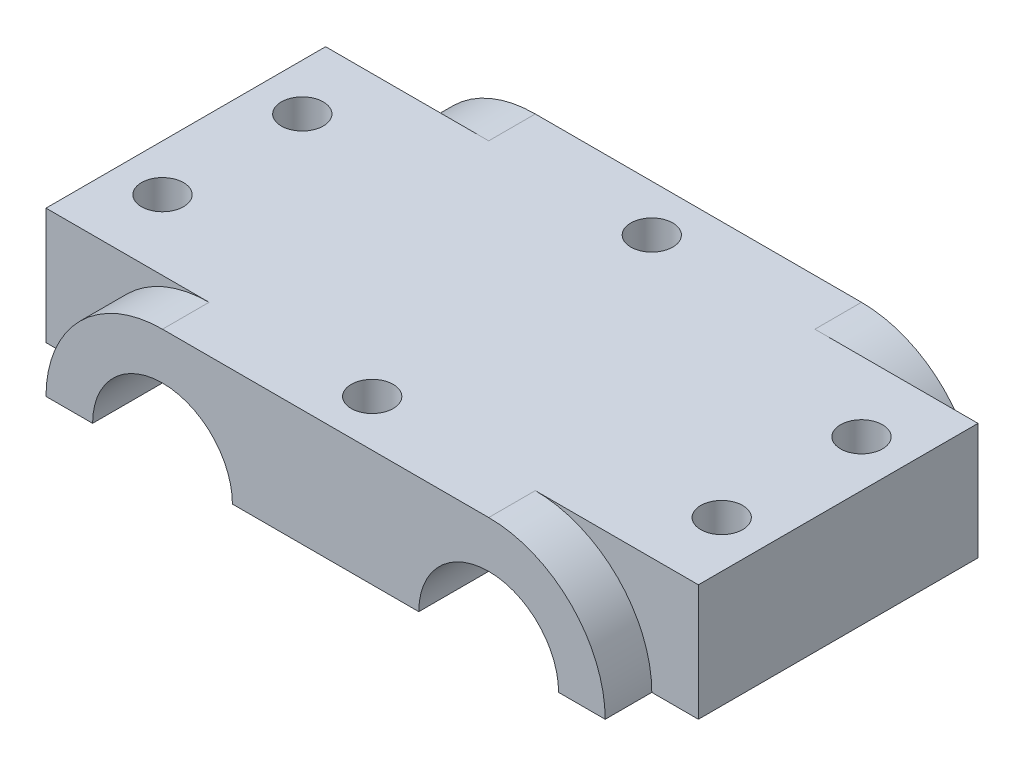
from build123d import *

# Parameters (mm, degrees)
BASE_BLOCK_PROFILE_SKETCH_W            = 70
BASE_BLOCK_PROFILE_SKETCH_H            = 12.5
BASE_BLOCK_DEPTH                       = 20
SADDLE_CUTOUTS_SKETCH_OUTSIDE_W        = 88.318
SADDLE_CUTOUTS_SKETCH_OUTSIDE_H        = 58.318
SADDLE_CUTOUTS_DEPTH                   = 40
MOUNTING_HOLES_4_5_SKETCH_R            = 2.25
MOUNTING_HOLES_4_5_SET_A_DEPTH         = 43.20485754
COLLAR_BOSS_DEPTH                      = 40
COLLAR_BORE_CUT_DEPTH                  = 54.516936583
CORNER_NOTCH_DEPTH                     = 5
CORNER_NOTCH_MIRROR_RIGHT_COPY_1_DEPTH = 5
COLLAR_TRIM_CUT_DEPTH                  = 50.890505121
COLLAR_RELIEF_SKETCH_R                 = 7.5
COLLAR_RELIEF_CUT_DEPTH                = 54.516936583
SKETCH6_2_R                            = 2.25
MOUNTING_HOLES_4_5_SET_B_DEPTH         = 43.20485757


with BuildPart() as part:
    # Base Block Profile Sketch → Base Block (new, symmetric)
    with BuildSketch(Plane.XY):
        Rectangle(BASE_BLOCK_PROFILE_SKETCH_W, BASE_BLOCK_PROFILE_SKETCH_H)
    extrude(amount=BASE_BLOCK_DEPTH, both=True)

    # Saddle Cutouts Sketch outside → Saddle Cutouts (cut)
    with BuildSketch(Plane(origin=(0, 6.25, 0), x_dir=(1, 0, 0), z_dir=(0, 1, 0))):
        Rectangle(SADDLE_CUTOUTS_SKETCH_OUTSIDE_W, SADDLE_CUTOUTS_SKETCH_OUTSIDE_H)
        Polygon((-22.5, 20), (-22.5, 15), (-35, 15), (-35, -15), (-22.5, -15), (-22.5, -20), (22.5, -20), (22.5, -15), (35, -15), (35, 15), (22.5, 15), (22.5, 20), align=None, mode=Mode.SUBTRACT)
    extrude(amount=-SADDLE_CUTOUTS_DEPTH, mode=Mode.SUBTRACT)

    # Mounting Holes _4.5 Sketch → Mounting Holes _4.5 Set A (cut, through all)
    with BuildSketch(Plane(origin=(0, 6.25, 0), x_dir=(1, 0, 0), z_dir=(0, 1, 0))):
        with Locations(Location((-30, 7.5, 0), (0, 0, 180))):
            Circle(MOUNTING_HOLES_4_5_SKETCH_R)
        with Locations(Location((-30, -7.5, 0), (0, 0, 180))):
            Circle(MOUNTING_HOLES_4_5_SKETCH_R)
        with Locations((30, -7.5)):
            Circle(MOUNTING_HOLES_4_5_SKETCH_R)
        with Locations((30, 7.5)):
            Circle(MOUNTING_HOLES_4_5_SKETCH_R)
        with Locations(Location((0, -15, 0), (0, 0, 180))):
            Circle(MOUNTING_HOLES_4_5_SKETCH_R)
        with Locations((0, 15)):
            Circle(MOUNTING_HOLES_4_5_SKETCH_R)
    extrude(amount=-MOUNTING_HOLES_4_5_SET_A_DEPTH, mode=Mode.SUBTRACT)

    # Collar Boss Sketch → Collar Boss (add, through all)
    with BuildSketch(Plane.XY.offset(20)):
        with BuildLine():
            Line((-30, -6.25), (-25, -6.25))
            ThreePointArc((-25, -6.25), (-17.5, 1.25), (-10, -6.25))
            Line((-10, -6.25), (-5, -6.25))
            ThreePointArc((-5, -6.25), (-17.5, 6.25), (-30, -6.25))
        make_face()
    collar_boss = extrude(amount=-COLLAR_BOSS_DEPTH)

    # Sketch7_2 → Collar Bore Cut (cut, through all)
    with BuildSketch(Plane.XY.offset(20)):
        with BuildLine():
            ThreePointArc((-10, -6.25), (-14.438137822, 0.596531969), (-22.5, -0.659830056))
            Line((-22.5, -0.659830056), (-22.5, -6.25))
            Line((-22.5, -6.25), (-10, -6.25))
        make_face()
    extrude(amount=-COLLAR_BORE_CUT_DEPTH, mode=Mode.SUBTRACT)

    # Corner Notch Sketch → Corner Notch (cut)
    with BuildSketch(Plane.XY.offset(20)):
        with BuildLine():
            Line((-22.5, 5.206439237), (-22.5, 6.25))
            Line((-22.5, 6.25), (-17.5, 6.25))
            ThreePointArc((-17.5, 6.25), (-20.053870546, 5.986328912), (-22.5, 5.206439237))
        make_face()
    corner_notch = extrude(amount=-CORNER_NOTCH_DEPTH, mode=Mode.SUBTRACT)

    # Corner Notch Mirror Front: Corner Notch across plane
    add(corner_notch.mirror(Plane.XY), mode=Mode.SUBTRACT)

    # Corner Notch Mirror Right: Corner Notch across plane
    add(corner_notch.mirror(Plane(origin=(0, 0, 0), x_dir=(0, 0, 1), z_dir=(1, 0, 0))), mode=Mode.SUBTRACT)

    # Corner Notch Mirror Right copy 1 sketch → Corner Notch Mirror Right copy 1 (cut)
    with BuildSketch(Plane(origin=(0, 0, -20), x_dir=(-1, 0, 0), z_dir=(0, 0, -1))):
        with BuildLine():
            Line((-22.5, 5.206439237), (-22.5, 6.25))
            Line((-22.5, 6.25), (-17.5, 6.25))
            ThreePointArc((-17.5, 6.25), (-20.053870546, 5.986328912), (-22.5, 5.206439237))
        make_face()
    extrude(amount=-CORNER_NOTCH_MIRROR_RIGHT_COPY_1_DEPTH, mode=Mode.SUBTRACT)

    # Collar Boss Mirror: Collar Boss across plane
    add(collar_boss.mirror(Plane(origin=(0, 0, 0), x_dir=(0, 0, 1), z_dir=(1, 0, 0))))

    # Collar Trim Sketch → Collar Trim Cut (cut, through all)
    with BuildSketch(Plane.XY.offset(15)):
        with BuildLine():
            Line((-25, -6.25), (-22.5, -6.25))
            Line((-22.5, -6.25), (-22.5, -0.659830056))
            ThreePointArc((-22.5, -0.659830056), (-24.346531969, -3.188137822), (-25, -6.25))
        make_face()
    extrude(amount=-COLLAR_TRIM_CUT_DEPTH, mode=Mode.SUBTRACT)

    # Collar Relief Sketch → Collar Relief Cut (cut, through all)
    with BuildSketch(Plane.XY.offset(20)):
        with Locations((17.5, -6.25)):
            Circle(COLLAR_RELIEF_SKETCH_R)
    extrude(amount=-COLLAR_RELIEF_CUT_DEPTH, mode=Mode.SUBTRACT)

    # Sketch6_2 → Mounting Holes _4.5 Set B (cut, through all)
    with BuildSketch(Plane(origin=(0, 6.25, 0), x_dir=(1, 0, 0), z_dir=(0, 1, 0))):
        with Locations(Location((-30, 7.5, 0), (0, 0, 180))):
            Circle(SKETCH6_2_R)
        with Locations(Location((-30, -7.5, 0), (0, 0, 180))):
            Circle(SKETCH6_2_R)
        with Locations((30, -7.5)):
            Circle(SKETCH6_2_R)
        with Locations((30, 7.5)):
            Circle(SKETCH6_2_R)
        with Locations(Location((0, -15, 0), (0, 0, 180))):
            Circle(SKETCH6_2_R)
        with Locations((0, 15)):
            Circle(SKETCH6_2_R)
    extrude(amount=-MOUNTING_HOLES_4_5_SET_B_DEPTH, mode=Mode.SUBTRACT)


solid = part.part
